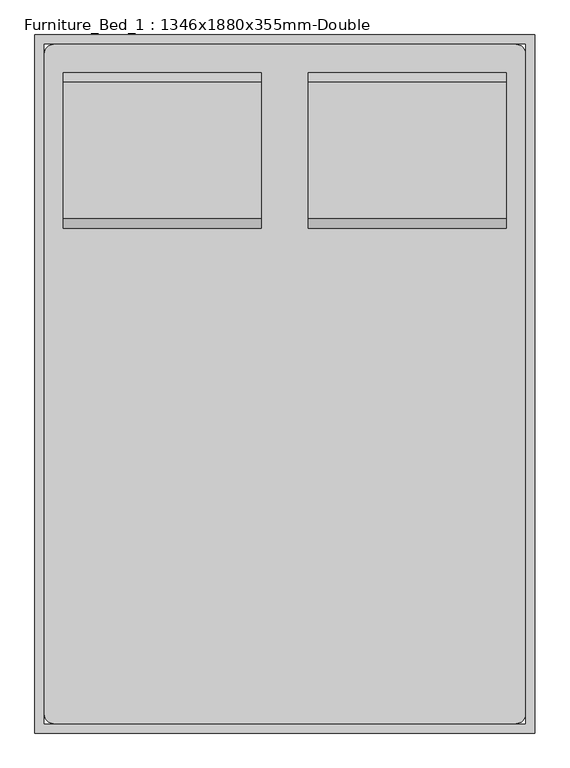
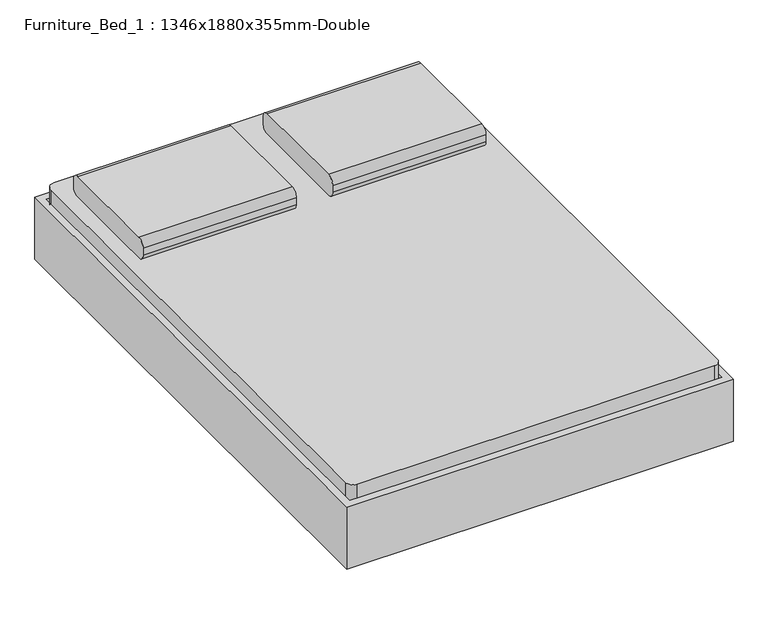
"""IFC4 building model written with IfcOpenShell, lengths in millimetres: furniture geometry, Furniture_Bed_1 : 1346x1880x355mm-Double."""

from ifc_helpers import new_model, si_unit, point, frame, frame_2d, origin, place, context, project, spatial, polyline, circle_curve, trimmed, segment, composite_curve, outline, extrude, source, transform, mapped, element, save
from ifc_brep_helpers import plane_surface, cylinder_surface, revolved_surface, advanced_brep


def furniture_bed_1_1346x1880x355mm_double_93dec6ea(model_context):
    return source(origin(), model_context, "Body", "SolidModel", [
        advanced_brep(
        [(-308.447541, -869.6295082, 196.85), (-308.447541, -869.6295082, 177.8), (-308.447541, -945.8295082, 177.8), (-308.447541, -945.8295082, 196.85), (-245.5113525, -869.6295082, 196.85), (-257.647541, -869.6295082, 177.8), (-257.647541, -945.8295082, 177.8), (-245.5113525, -945.8295082, 196.85), (-164.3115092, -869.6295082, 22.716374), (-181.5766725, -869.6295082, 14.6654962), (-181.5766725, -945.8295082, 14.6654962), (-164.3115092, -945.8295082, 22.716374), (-158.5564547, -869.6295082, 0.0), (-158.5564547, -869.6295082, 19.05), (-158.5564547, -945.8295082, 0.0), (-158.5564547, -945.8295082, 19.05), (-79.9439489, -869.6295082, 19.05), (-79.9439489, -869.6295082, 0.0), (-79.9439489, -945.8295082, 0.0), (-79.9439489, -945.8295082, 19.05), (-67.2439489, -869.6295082, 3.4029547), (-76.7689489, -869.6295082, 19.9007387), (-67.2439489, -945.8295082, 3.4029547), (-76.7689489, -945.8295082, 19.9007387), (-12.2513357, -869.6295082, 57.15), (-7.1469036, -869.6295082, 38.1), (-7.1469036, -945.8295082, 38.1), (-12.2513357, -945.8295082, 57.15), (690.5562537, -869.6295082, 57.15), (685.4518216, -869.6295082, 38.1), (685.4518216, -945.8295082, 38.1), (690.5562537, -945.8295082, 57.15), (755.0738669, -869.6295082, 19.9007387), (745.5488669, -869.6295082, 3.4029547), (745.5488669, -945.8295082, 3.4029547), (755.0738669, -945.8295082, 19.9007387), (758.2488669, -869.6295082, 0.0), (758.2488669, -869.6295082, 19.05), (758.2488669, -945.8295082, 0.0), (758.2488669, -945.8295082, 19.05), (836.8613728, -869.6295082, 19.05), (836.8613728, -869.6295082, 0.0), (836.8613728, -945.8295082, 0.0), (836.8613728, -945.8295082, 19.05), (859.8815906, -869.6295082, 14.6654962), (842.6164272, -869.6295082, 22.716374), (859.8815906, -945.8295082, 14.6654962), (842.6164272, -945.8295082, 22.716374), (923.8162705, -869.6295082, 196.85), (935.952459, -869.6295082, 177.8), (935.952459, -945.8295082, 177.8), (923.8162705, -945.8295082, 196.85), (986.752459, -869.6295082, 196.85), (986.752459, -945.8295082, 196.85), (986.752459, -945.8295082, 177.8), (986.752459, -869.6295082, 177.8)],
        [
            (0, 1),
            (1, 2),
            (2, 3),
            (3, 0),
            (0, 4),
            (4, 5),
            (5, 1),
            (5, 6),
            (6, 2),
            (6, 7),
            (7, 3),
            (7, 4),
            (4, 8),
            (8, 9),
            (9, 5),
            (9, 10),
            (10, 6),
            (10, 11),
            (11, 7),
            (11, 8),
            (12, 9, circle_curve(frame((-158.5564547, -869.6295082, 25.4), z_axis=(0.0, 1.0, 0.0), x_axis=(-0.9063077870366627, 0.0, -0.42261826174067213)), 25.4)),
            (8, 13, circle_curve(frame((-158.5564547, -869.6295082, 25.4), z_axis=(0.0, -1.0, 0.0), x_axis=(-0.9063077870366627, 0.0, -0.42261826174067213)), 6.35)),
            (13, 12),
            (14, 10, circle_curve(frame((-158.5564547, -945.8295082, 25.4), z_axis=(0.0, 1.0, 0.0), x_axis=(-0.9063077870366627, 0.0, -0.42261826174067213)), 25.4)),
            (12, 14),
            (15, 11, circle_curve(frame((-158.5564547, -945.8295082, 25.4), z_axis=(0.0, 1.0, 0.0), x_axis=(-0.9063077870366627, 0.0, -0.42261826174067213)), 6.35)),
            (14, 15),
            (15, 13),
            (13, 16),
            (16, 17),
            (17, 12),
            (17, 18),
            (18, 14),
            (18, 19),
            (19, 15),
            (19, 16),
            (20, 17, circle_curve(frame((-79.9439489, -869.6295082, 25.4), z_axis=(0.0, 1.0, 0.0), x_axis=(0.0, 0.0, -1.0)), 25.4)),
            (16, 21, circle_curve(frame((-79.9439489, -869.6295082, 25.4), z_axis=(0.0, -1.0, 0.0), x_axis=(0.0, 0.0, -1.0)), 6.35)),
            (21, 20),
            (22, 18, circle_curve(frame((-79.9439489, -945.8295082, 25.4), z_axis=(0.0, 1.0, 0.0), x_axis=(0.0, 0.0, -1.0)), 25.4)),
            (20, 22),
            (23, 19, circle_curve(frame((-79.9439489, -945.8295082, 25.4), z_axis=(0.0, 1.0, 0.0), x_axis=(0.0, 0.0, -1.0)), 6.35)),
            (22, 23),
            (23, 21),
            (21, 24),
            (24, 25),
            (25, 20),
            (25, 26),
            (26, 22),
            (26, 27),
            (27, 23),
            (27, 24),
            (24, 28),
            (28, 29),
            (29, 25),
            (29, 30),
            (30, 26),
            (30, 31),
            (31, 27),
            (31, 28),
            (28, 32),
            (32, 33),
            (33, 29),
            (33, 34),
            (34, 30),
            (34, 35),
            (35, 31),
            (35, 32),
            (36, 33, circle_curve(frame((758.2488669, -869.6295082, 25.4), z_axis=(0.0, 1.0, 0.0), x_axis=(-0.5000000000000486, 0.0, -0.8660254037844105)), 25.4)),
            (32, 37, circle_curve(frame((758.2488669, -869.6295082, 25.4), z_axis=(0.0, -1.0, 0.0), x_axis=(-0.5000000000000486, 0.0, -0.8660254037844105)), 6.35)),
            (37, 36),
            (38, 34, circle_curve(frame((758.2488669, -945.8295082, 25.4), z_axis=(0.0, 1.0, 0.0), x_axis=(-0.5000000000000486, 0.0, -0.8660254037844105)), 25.4)),
            (36, 38),
            (39, 35, circle_curve(frame((758.2488669, -945.8295082, 25.4), z_axis=(0.0, 1.0, 0.0), x_axis=(-0.5000000000000486, 0.0, -0.8660254037844105)), 6.35)),
            (38, 39),
            (39, 37),
            (37, 40),
            (40, 41),
            (41, 36),
            (41, 42),
            (42, 38),
            (42, 43),
            (43, 39),
            (43, 40),
            (44, 41, circle_curve(frame((836.8613728, -869.6295082, 25.4), z_axis=(0.0, 1.0, 0.0), x_axis=(0.0, 0.0, -1.0)), 25.4)),
            (40, 45, circle_curve(frame((836.8613728, -869.6295082, 25.4), z_axis=(0.0, -1.0, 0.0), x_axis=(0.0, 0.0, -1.0)), 6.35)),
            (45, 44),
            (46, 42, circle_curve(frame((836.8613728, -945.8295082, 25.4), z_axis=(0.0, 1.0, 0.0), x_axis=(0.0, 0.0, -1.0)), 25.4)),
            (44, 46),
            (47, 43, circle_curve(frame((836.8613728, -945.8295082, 25.4), z_axis=(0.0, 1.0, 0.0), x_axis=(0.0, 0.0, -1.0)), 6.35)),
            (46, 47),
            (47, 45),
            (45, 48),
            (48, 49),
            (49, 44),
            (49, 50),
            (50, 46),
            (50, 51),
            (51, 47),
            (51, 48),
            (52, 53),
            (53, 54),
            (54, 55),
            (55, 52),
            (48, 52),
            (55, 49),
            (54, 50),
            (53, 51),
        ],
        [
            plane_surface(frame((-308.447541, -1174.4295082, -127.5947323), z_axis=(-1.0, 0.0, 0.0), x_axis=(0.0, 1.0, 0.0))),
            plane_surface(frame((-308.447541, -869.6295082, 196.85), z_axis=(0.0, 1.0, 0.0), x_axis=(1.0, 0.0, 0.0))),
            plane_surface(frame((-308.447541, -869.6295082, 177.8), z_axis=(0.0, 0.0, -1.0), x_axis=(1.0, 0.0, 0.0))),
            plane_surface(frame((-308.447541, -945.8295082, 177.8), z_axis=(0.0, -1.0, 0.0), x_axis=(1.0, 0.0, 0.0))),
            plane_surface(frame((-308.447541, -945.8295082, 196.85), z_axis=(0.0, 0.0, 1.0), x_axis=(1.0, 0.0, 0.0))),
            plane_surface(frame((-245.5113525, -869.6295082, 196.85), z_axis=(0.0, 1.0, 0.0), x_axis=(0.42261826174067146, 0.0, -0.906307787036663))),
            plane_surface(frame((-257.647541, -869.6295082, 177.8), z_axis=(-0.9063077870366631, 0.0, -0.4226182617406713), x_axis=(0.4226182617406713, 0.0, -0.9063077870366631))),
            plane_surface(frame((-257.647541, -945.8295082, 177.8), z_axis=(0.0, -1.0, 0.0), x_axis=(0.4226182617406716, 0.0, -0.9063077870366629))),
            plane_surface(frame((-245.5113525, -945.8295082, 196.85), z_axis=(0.906307787036663, 0.0, 0.4226182617406716), x_axis=(0.4226182617406716, 0.0, -0.906307787036663))),
            plane_surface(frame((-158.5564547, -869.6295082, 25.4), z_axis=(0.0, 1.0, 0.0), x_axis=(-0.9063077870366627, 0.0, -0.42261826174067213))),
            cylinder_surface(frame((-158.5564547, -1174.4295082, 25.4), z_axis=(0.0, -1.0, 0.0), x_axis=(-0.9063077870366627, 0.0, -0.42261826174067213)), 25.4),
            plane_surface(frame((-158.5564547, -945.8295082, 25.4), z_axis=(0.0, -1.0, 0.0), x_axis=(-0.9063077870366627, 0.0, -0.42261826174067213))),
            revolved_surface(polyline([(-164.31150914768278, -945.8295082, 22.716374037946732), (-164.31150914768278, -869.6295082, 22.716374037946732)]), (-158.5564547, -1174.4295082, 25.4), (0.0, -1.0, 0.0)),
            plane_surface(frame((-158.5564547, -869.6295082, 19.05), z_axis=(0.0, 1.0, 0.0), x_axis=(1.0, 0.0, 0.0))),
            plane_surface(frame((-158.5564547, -869.6295082, 0.0), z_axis=(0.0, 0.0, -1.0), x_axis=(1.0, 0.0, 0.0))),
            plane_surface(frame((-158.5564547, -945.8295082, 0.0), z_axis=(0.0, -1.0, 0.0), x_axis=(1.0, 0.0, 0.0))),
            plane_surface(frame((-158.5564547, -945.8295082, 19.05), z_axis=(0.0, 0.0, 1.0), x_axis=(1.0, 0.0, 0.0))),
            plane_surface(frame((-79.9439489, -869.6295082, 25.4), z_axis=(0.0, 1.0, 0.0), x_axis=(0.0, 0.0, -1.0))),
            cylinder_surface(frame((-79.9439489, -1174.4295082, 25.4), z_axis=(0.0, -1.0, 0.0), x_axis=(0.0, 0.0, -1.0)), 25.4),
            plane_surface(frame((-79.9439489, -945.8295082, 25.4), z_axis=(0.0, -1.0, 0.0), x_axis=(0.0, 0.0, -1.0))),
            revolved_surface(polyline([(-79.9439489, -945.8295082, 19.049999999999997), (-79.9439489, -869.6295082, 19.049999999999997)]), (-79.9439489, -1174.4295082, 25.4), (0.0, -1.0, 0.0)),
            plane_surface(frame((-76.7689489, -869.6295082, 19.9007387), z_axis=(0.0, 1.0, 0.0), x_axis=(0.8660254037844782, 0.0, 0.4999999999999314))),
            plane_surface(frame((-67.2439489, -869.6295082, 3.4029547), z_axis=(0.49999999999993133, 0.0, -0.8660254037844783), x_axis=(0.8660254037844783, 0.0, 0.49999999999993133))),
            plane_surface(frame((-67.2439489, -945.8295082, 3.4029547), z_axis=(0.0, -1.0, 0.0), x_axis=(0.8660254037844785, 0.0, 0.499999999999931))),
            plane_surface(frame((-76.7689489, -945.8295082, 19.9007387), z_axis=(-0.49999999999993144, 0.0, 0.8660254037844782), x_axis=(0.8660254037844782, 0.0, 0.49999999999993144))),
            plane_surface(frame((-12.2513357, -869.6295082, 57.15), z_axis=(0.0, 1.0, 0.0), x_axis=(1.0, 0.0, 0.0))),
            plane_surface(frame((-7.1469036, -869.6295082, 38.1), z_axis=(0.0, 0.0, -1.0), x_axis=(1.0, 0.0, 0.0))),
            plane_surface(frame((-7.1469036, -945.8295082, 38.1), z_axis=(0.0, -1.0, 0.0), x_axis=(1.0, 0.0, 0.0))),
            plane_surface(frame((-12.2513357, -945.8295082, 57.15), z_axis=(0.0, 0.0, 1.0), x_axis=(1.0, 0.0, 0.0))),
            plane_surface(frame((690.5562537, -869.6295082, 57.15), z_axis=(0.0, 1.0, 0.0), x_axis=(0.8660254037844104, 0.0, -0.5000000000000491))),
            plane_surface(frame((685.4518216, -869.6295082, 38.1), z_axis=(-0.5000000000000484, 0.0, -0.8660254037844108), x_axis=(0.8660254037844108, 0.0, -0.5000000000000484))),
            plane_surface(frame((685.4518216, -945.8295082, 38.1), z_axis=(0.0, -1.0000000000000002, 0.0), x_axis=(0.8660254037844103, 0.0, -0.5000000000000493))),
            plane_surface(frame((690.5562537, -945.8295082, 57.15), z_axis=(0.5000000000000485, 0.0, 0.8660254037844106), x_axis=(0.8660254037844106, 0.0, -0.5000000000000485))),
            plane_surface(frame((758.2488669, -869.6295082, 25.4), z_axis=(0.0, 1.0000000000000002, 0.0), x_axis=(-0.5000000000000487, 0.0, -0.8660254037844106))),
            cylinder_surface(frame((758.2488669, -1174.4295082, 25.4), z_axis=(0.0, -1.0, 0.0), x_axis=(-0.5000000000000486, 0.0, -0.8660254037844105)), 25.4),
            plane_surface(frame((758.2488669, -945.8295082, 25.4), z_axis=(0.0, -1.0000000000000002, 0.0), x_axis=(-0.5000000000000487, 0.0, -0.8660254037844106))),
            revolved_surface(polyline([(755.0738668999998, -945.8295082, 19.900738685968992), (755.0738668999998, -869.6295082, 19.900738685968992)]), (758.2488669, -1174.4295082, 25.4), (0.0, -1.0, 0.0)),
            plane_surface(frame((758.2488669, -869.6295082, 19.05), z_axis=(0.0, 1.0, 0.0), x_axis=(1.0, 0.0, 0.0))),
            plane_surface(frame((758.2488669, -869.6295082, 0.0), z_axis=(0.0, 0.0, -1.0), x_axis=(1.0, 0.0, 0.0))),
            plane_surface(frame((758.2488669, -945.8295082, 0.0), z_axis=(0.0, -1.0, 0.0), x_axis=(1.0, 0.0, 0.0))),
            plane_surface(frame((758.2488669, -945.8295082, 19.05), z_axis=(0.0, 0.0, 1.0), x_axis=(1.0, 0.0, 0.0))),
            plane_surface(frame((836.8613728, -869.6295082, 25.4), z_axis=(0.0, 1.0, 0.0), x_axis=(0.0, 0.0, -1.0))),
            cylinder_surface(frame((836.8613728, -1174.4295082, 25.4), z_axis=(0.0, -1.0, 0.0), x_axis=(0.0, 0.0, -1.0)), 25.4),
            plane_surface(frame((836.8613728, -945.8295082, 25.4), z_axis=(0.0, -1.0, 0.0), x_axis=(0.0, 0.0, -1.0))),
            revolved_surface(polyline([(836.8613728, -945.8295082, 19.049999999999997), (836.8613728, -869.6295082, 19.049999999999997)]), (836.8613728, -1174.4295082, 25.4), (0.0, -1.0, 0.0)),
            plane_surface(frame((842.6164272, -869.6295082, 22.716374), z_axis=(0.0, 1.0, 0.0), x_axis=(0.4226182617405402, 0.0, 0.9063077870367242))),
            plane_surface(frame((859.8815906, -869.6295082, 14.6654962), z_axis=(0.9063077870367245, 0.0, -0.42261826174053974), x_axis=(0.42261826174053974, 0.0, 0.9063077870367245))),
            plane_surface(frame((859.8815906, -945.8295082, 14.6654962), z_axis=(0.0, -1.0000000000000002, 0.0), x_axis=(0.42261826174053974, 0.0, 0.9063077870367245))),
            plane_surface(frame((842.6164272, -945.8295082, 22.716374), z_axis=(-0.9063077870367247, 0.0, 0.4226182617405394), x_axis=(0.4226182617405394, 0.0, 0.9063077870367247))),
            plane_surface(frame((986.752459, -1174.4295082, -127.5947323), z_axis=(1.0, 0.0, 0.0), x_axis=(0.0, 1.0, 0.0))),
            plane_surface(frame((923.8162705, -869.6295082, 196.85), z_axis=(0.0, 1.0, 0.0), x_axis=(1.0, 0.0, 0.0))),
            plane_surface(frame((935.952459, -869.6295082, 177.8), z_axis=(0.0, 0.0, -1.0), x_axis=(1.0, 0.0, 0.0))),
            plane_surface(frame((935.952459, -945.8295082, 177.8), z_axis=(0.0, -1.0, 0.0), x_axis=(1.0, 0.0, 0.0))),
            plane_surface(frame((923.8162705, -945.8295082, 196.85), z_axis=(0.0, 0.0, 1.0), x_axis=(1.0, 0.0, 0.0))),
        ],
        [
            (0, [[1, 2, 3, 4]]),
            (1, [[-1, 5, 6, 7]]),
            (2, [[-2, -7, 8, 9]]),
            (3, [[-3, -9, 10, 11]]),
            (4, [[-4, -11, 12, -5]]),
            (5, [[-6, 13, 14, 15]]),
            (6, [[-8, -15, 16, 17]]),
            (7, [[-10, -17, 18, 19]]),
            (8, [[-12, -19, 20, -13]]),
            (9, [[21, -14, 22, 23]]),
            (10, [[24, -16, -21, 25]]),
            (11, [[26, -18, -24, 27]]),
            (12, [[-22, -20, -26, 28]]),
            (13, [[-23, 29, 30, 31]]),
            (14, [[-25, -31, 32, 33]]),
            (15, [[-27, -33, 34, 35]]),
            (16, [[-28, -35, 36, -29]]),
            (17, [[37, -30, 38, 39]]),
            (18, [[40, -32, -37, 41]]),
            (19, [[42, -34, -40, 43]]),
            (20, [[-38, -36, -42, 44]]),
            (21, [[-39, 45, 46, 47]]),
            (22, [[-41, -47, 48, 49]]),
            (23, [[-43, -49, 50, 51]]),
            (24, [[-44, -51, 52, -45]]),
            (25, [[-46, 53, 54, 55]]),
            (26, [[-48, -55, 56, 57]]),
            (27, [[-50, -57, 58, 59]]),
            (28, [[-52, -59, 60, -53]]),
            (29, [[-54, 61, 62, 63]]),
            (30, [[-56, -63, 64, 65]]),
            (31, [[-58, -65, 66, 67]]),
            (32, [[-60, -67, 68, -61]]),
            (33, [[69, -62, 70, 71]]),
            (34, [[72, -64, -69, 73]]),
            (35, [[74, -66, -72, 75]]),
            (36, [[-70, -68, -74, 76]]),
            (37, [[-71, 77, 78, 79]]),
            (38, [[-73, -79, 80, 81]]),
            (39, [[-75, -81, 82, 83]]),
            (40, [[-76, -83, 84, -77]]),
            (41, [[85, -78, 86, 87]]),
            (42, [[88, -80, -85, 89]]),
            (43, [[90, -82, -88, 91]]),
            (44, [[-86, -84, -90, 92]]),
            (45, [[-87, 93, 94, 95]]),
            (46, [[-89, -95, 96, 97]]),
            (47, [[-91, -97, 98, 99]]),
            (48, [[-92, -99, 100, -93]]),
            (49, [[101, 102, 103, 104]]),
            (50, [[-94, 105, -104, 106]]),
            (51, [[-96, -106, -103, 107]]),
            (52, [[-98, -107, -102, 108]]),
            (53, [[-100, -108, -101, -105]]),
        ],
    ),
        extrude(outline(composite_curve([segment(polyline([(-283.047541, 680.1704918), (961.352459, 680.1704918)]), True, "CONTINUOUS"), segment(trimmed(circle_curve(frame_2d((961.352459, 654.7704918)), 25.4), [point((961.352459, 680.1704918))], [point((986.752459, 654.7704918))], False, "CARTESIAN"), True, "CONTINUOUS"), segment(polyline([(986.752459, 654.7704918), (986.752459, -1123.6295082)]), True, "CONTINUOUS"), segment(trimmed(circle_curve(frame_2d((961.352459, -1123.6295082)), 25.4), [point((986.752459, -1123.6295082))], [point((961.352459, -1149.0295082))], False, "CARTESIAN"), True, "CONTINUOUS"), segment(polyline([(961.352459, -1149.0295082), (-283.047541, -1149.0295082)]), True, "CONTINUOUS"), segment(trimmed(circle_curve(frame_2d((-283.047541, -1123.6295082)), 25.4), [point((-283.047541, -1149.0295082))], [point((-308.447541, -1123.6295082))], False, "CARTESIAN"), True, "CONTINUOUS"), segment(polyline([(-308.447541, -1123.6295082), (-308.447541, 654.7704918)]), True, "CONTINUOUS"), segment(trimmed(circle_curve(frame_2d((-283.047541, 654.7704918)), 25.4), [point((-308.447541, 654.7704918))], [point((-283.047541, 680.1704918))], False, "CARTESIAN"), True, "CONTINUOUS")], self_intersect=False)), frame((0.0, 0.0, 203.2), z_axis=(0.0, 0.0, 1.0), x_axis=(1.0, 0.0, 0.0)), (0.0, 0.0, 1.0), 203.2),
        advanced_brep(
        [(-308.1231784, 451.5704918, 177.8), (-308.1231784, 375.3704918, 177.8), (-308.1231784, 375.3704918, 196.85), (-308.1231784, 451.5704918, 196.85), (-257.3231784, 451.5704918, 177.8), (-257.3231784, 375.3704918, 177.8), (-245.1869899, 375.3704918, 196.85), (-245.1869899, 451.5704918, 196.85), (-181.2523099, 451.5704918, 14.6654962), (-181.2523099, 375.3704918, 14.6654962), (-163.9871466, 375.3704918, 22.716374), (-163.9871466, 451.5704918, 22.716374), (-158.2320921, 375.3704918, 0.0), (-158.2320921, 451.5704918, 0.0), (-158.2320921, 375.3704918, 19.05), (-158.2320921, 451.5704918, 19.05), (-79.6195862, 451.5704918, 0.0), (-79.6195862, 375.3704918, 0.0), (-79.6195862, 375.3704918, 19.05), (-79.6195862, 451.5704918, 19.05), (-66.9195862, 375.3704918, 3.4029547), (-66.9195862, 451.5704918, 3.4029547), (-76.4445862, 375.3704918, 19.9007387), (-76.4445862, 451.5704918, 19.9007387), (-6.822541, 451.5704918, 38.1), (-6.822541, 375.3704918, 38.1), (-11.9269731, 375.3704918, 57.15), (-11.9269731, 451.5704918, 57.15), (685.4518216, 451.5704918, 38.1), (685.4518216, 375.3704918, 38.1), (690.5562537, 375.3704918, 57.15), (690.5562537, 451.5704918, 57.15), (745.5488669, 451.5704918, 3.4029547), (745.5488669, 375.3704918, 3.4029547), (755.0738669, 375.3704918, 19.9007387), (755.0738669, 451.5704918, 19.9007387), (758.2488669, 375.3704918, 0.0), (758.2488669, 451.5704918, 0.0), (758.2488669, 375.3704918, 19.05), (758.2488669, 451.5704918, 19.05), (836.8613728, 451.5704918, 0.0), (836.8613728, 375.3704918, 0.0), (836.8613728, 375.3704918, 19.05), (836.8613728, 451.5704918, 19.05), (859.8815906, 375.3704918, 14.6654962), (859.8815906, 451.5704918, 14.6654962), (842.6164272, 375.3704918, 22.716374), (842.6164272, 451.5704918, 22.716374), (935.952459, 451.5704918, 177.8), (935.952459, 375.3704918, 177.8), (923.8162705, 375.3704918, 196.85), (923.8162705, 451.5704918, 196.85), (986.752459, 451.5704918, 177.8), (986.752459, 451.5704918, 196.85), (986.752459, 375.3704918, 196.85), (986.752459, 375.3704918, 177.8)],
        [
            (0, 1),
            (1, 2),
            (2, 3),
            (3, 0),
            (0, 4),
            (4, 5),
            (5, 1),
            (5, 6),
            (6, 2),
            (6, 7),
            (7, 3),
            (7, 4),
            (4, 8),
            (8, 9),
            (9, 5),
            (9, 10),
            (10, 6),
            (10, 11),
            (11, 7),
            (11, 8),
            (12, 9, circle_curve(frame((-158.2320921, 375.3704918, 25.4), z_axis=(0.0, 1.0, 0.0), x_axis=(-0.906307787036649, 0.0, -0.4226182617407015)), 25.4)),
            (8, 13, circle_curve(frame((-158.2320921, 451.5704918, 25.4), z_axis=(0.0, -1.0, 0.0), x_axis=(-0.906307787036649, 0.0, -0.4226182617407015)), 25.4)),
            (13, 12),
            (14, 10, circle_curve(frame((-158.2320921, 375.3704918, 25.4), z_axis=(0.0, 1.0, 0.0), x_axis=(-0.906307787036649, 0.0, -0.4226182617407015)), 6.35)),
            (12, 14),
            (15, 11, circle_curve(frame((-158.2320921, 451.5704918, 25.4), z_axis=(0.0, 1.0, 0.0), x_axis=(-0.906307787036649, 0.0, -0.4226182617407015)), 6.35)),
            (14, 15),
            (15, 13),
            (13, 16),
            (16, 17),
            (17, 12),
            (17, 18),
            (18, 14),
            (18, 19),
            (19, 15),
            (19, 16),
            (20, 17, circle_curve(frame((-79.6195862, 375.3704918, 25.4), z_axis=(0.0, 1.0, 0.0), x_axis=(0.0, 0.0, -1.0)), 25.4)),
            (16, 21, circle_curve(frame((-79.6195862, 451.5704918, 25.4), z_axis=(0.0, -1.0, 0.0), x_axis=(0.0, 0.0, -1.0)), 25.4)),
            (21, 20),
            (22, 18, circle_curve(frame((-79.6195862, 375.3704918, 25.4), z_axis=(0.0, 1.0, 0.0), x_axis=(0.0, 0.0, -1.0)), 6.35)),
            (20, 22),
            (23, 19, circle_curve(frame((-79.6195862, 451.5704918, 25.4), z_axis=(0.0, 1.0, 0.0), x_axis=(0.0, 0.0, -1.0)), 6.35)),
            (22, 23),
            (23, 21),
            (21, 24),
            (24, 25),
            (25, 20),
            (25, 26),
            (26, 22),
            (26, 27),
            (27, 23),
            (27, 24),
            (24, 28),
            (28, 29),
            (29, 25),
            (29, 30),
            (30, 26),
            (30, 31),
            (31, 27),
            (31, 28),
            (28, 32),
            (32, 33),
            (33, 29),
            (33, 34),
            (34, 30),
            (34, 35),
            (35, 31),
            (35, 32),
            (36, 33, circle_curve(frame((758.2488669, 375.3704918, 25.4), z_axis=(0.0, 1.0, 0.0), x_axis=(-0.5000000000000444, 0.0, -0.866025403784413)), 25.4)),
            (32, 37, circle_curve(frame((758.2488669, 451.5704918, 25.4), z_axis=(0.0, -1.0, 0.0), x_axis=(-0.5000000000000444, 0.0, -0.866025403784413)), 25.4)),
            (37, 36),
            (38, 34, circle_curve(frame((758.2488669, 375.3704918, 25.4), z_axis=(0.0, 1.0, 0.0), x_axis=(-0.5000000000000444, 0.0, -0.866025403784413)), 6.35)),
            (36, 38),
            (39, 35, circle_curve(frame((758.2488669, 451.5704918, 25.4), z_axis=(0.0, 1.0, 0.0), x_axis=(-0.5000000000000444, 0.0, -0.866025403784413)), 6.35)),
            (38, 39),
            (39, 37),
            (37, 40),
            (40, 41),
            (41, 36),
            (41, 42),
            (42, 38),
            (42, 43),
            (43, 39),
            (43, 40),
            (44, 41, circle_curve(frame((836.8613728, 375.3704918, 25.4), z_axis=(0.0, 1.0, 0.0), x_axis=(0.0, 0.0, -1.0)), 25.4)),
            (40, 45, circle_curve(frame((836.8613728, 451.5704918, 25.4), z_axis=(0.0, -1.0, 0.0), x_axis=(0.0, 0.0, -1.0)), 25.4)),
            (45, 44),
            (46, 42, circle_curve(frame((836.8613728, 375.3704918, 25.4), z_axis=(0.0, 1.0, 0.0), x_axis=(0.0, 0.0, -1.0)), 6.35)),
            (44, 46),
            (47, 43, circle_curve(frame((836.8613728, 451.5704918, 25.4), z_axis=(0.0, 1.0, 0.0), x_axis=(0.0, 0.0, -1.0)), 6.35)),
            (46, 47),
            (47, 45),
            (45, 48),
            (48, 49),
            (49, 44),
            (49, 50),
            (50, 46),
            (50, 51),
            (51, 47),
            (51, 48),
            (52, 53),
            (53, 54),
            (54, 55),
            (55, 52),
            (48, 52),
            (55, 49),
            (54, 50),
            (53, 51),
        ],
        [
            plane_surface(frame((-308.1231784, 705.5704918, -152.9490627), z_axis=(-1.0, 0.0, 0.0), x_axis=(0.0, 1.0, 0.0))),
            plane_surface(frame((-308.1231784, 451.5704918, 177.8), z_axis=(0.0, 0.0, -1.0), x_axis=(1.0, 0.0, 0.0))),
            plane_surface(frame((-308.1231784, 375.3704918, 177.8), z_axis=(0.0, -1.0, 0.0), x_axis=(1.0, 0.0, 0.0))),
            plane_surface(frame((-308.1231784, 375.3704918, 196.85), z_axis=(0.0, 0.0, 1.0), x_axis=(1.0, 0.0, 0.0))),
            plane_surface(frame((-308.1231784, 451.5704918, 196.85), z_axis=(0.0, 1.0, 0.0), x_axis=(1.0, 0.0, 0.0))),
            plane_surface(frame((-257.3231784, 451.5704918, 177.8), z_axis=(-0.9063077870366483, 0.0, -0.4226182617407031), x_axis=(0.4226182617407031, 0.0, -0.9063077870366483))),
            plane_surface(frame((-257.3231784, 375.3704918, 177.8), z_axis=(0.0, -1.0, 0.0), x_axis=(0.4226182617407027, 0.0, -0.9063077870366485))),
            plane_surface(frame((-245.1869899, 375.3704918, 196.85), z_axis=(0.9063077870366484, 0.0, 0.4226182617407029), x_axis=(0.4226182617407029, 0.0, -0.9063077870366484))),
            plane_surface(frame((-245.1869899, 451.5704918, 196.85), z_axis=(0.0, 1.0, 0.0), x_axis=(0.4226182617407027, 0.0, -0.9063077870366485))),
            cylinder_surface(frame((-158.2320921, 705.5704918, 25.4), z_axis=(0.0, -1.0, 0.0), x_axis=(-0.906307787036649, 0.0, -0.4226182617407015)), 25.4),
            plane_surface(frame((-158.2320921, 375.3704918, 25.4), z_axis=(0.0, -1.0, 0.0), x_axis=(-0.906307787036649, 0.0, -0.4226182617407015))),
            revolved_surface(polyline([(-163.9871465476827, 375.3704918, 22.716374037946544), (-163.9871465476827, 451.5704918, 22.716374037946544)]), (-158.2320921, 705.5704918, 25.4), (0.0, -1.0, 0.0)),
            plane_surface(frame((-158.2320921, 451.5704918, 25.4), z_axis=(0.0, 1.0, 0.0), x_axis=(-0.906307787036649, 0.0, -0.4226182617407015))),
            plane_surface(frame((-158.2320921, 451.5704918, 0.0), z_axis=(0.0, 0.0, -1.0), x_axis=(1.0, 0.0, 0.0))),
            plane_surface(frame((-158.2320921, 375.3704918, 0.0), z_axis=(0.0, -1.0, 0.0), x_axis=(1.0, 0.0, 0.0))),
            plane_surface(frame((-158.2320921, 375.3704918, 19.05), z_axis=(0.0, 0.0, 1.0), x_axis=(1.0, 0.0, 0.0))),
            plane_surface(frame((-158.2320921, 451.5704918, 19.05), z_axis=(0.0, 1.0, 0.0), x_axis=(1.0, 0.0, 0.0))),
            cylinder_surface(frame((-79.6195862, 705.5704918, 25.4), z_axis=(0.0, -1.0, 0.0), x_axis=(0.0, 0.0, -1.0)), 25.4),
            plane_surface(frame((-79.6195862, 375.3704918, 25.4), z_axis=(0.0, -1.0, 0.0), x_axis=(0.0, 0.0, -1.0))),
            revolved_surface(polyline([(-79.6195862, 375.3704918, 19.049999999999997), (-79.6195862, 451.5704918, 19.049999999999997)]), (-79.6195862, 705.5704918, 25.4), (0.0, -1.0, 0.0)),
            plane_surface(frame((-79.6195862, 451.5704918, 25.4), z_axis=(0.0, 1.0, 0.0), x_axis=(0.0, 0.0, -1.0))),
            plane_surface(frame((-66.9195862, 451.5704918, 3.4029547), z_axis=(0.4999999999998771, 0.0, -0.8660254037845097), x_axis=(0.8660254037845097, 0.0, 0.4999999999998771))),
            plane_surface(frame((-66.9195862, 375.3704918, 3.4029547), z_axis=(0.0, -1.0000000000000002, 0.0), x_axis=(0.8660254037845102, 0.0, 0.49999999999987627))),
            plane_surface(frame((-76.4445862, 375.3704918, 19.9007387), z_axis=(-0.49999999999987643, 0.0, 0.86602540378451), x_axis=(0.86602540378451, 0.0, 0.49999999999987643))),
            plane_surface(frame((-76.4445862, 451.5704918, 19.9007387), z_axis=(0.0, 1.0, 0.0), x_axis=(0.8660254037845102, 0.0, 0.4999999999998761))),
            plane_surface(frame((-6.822541, 451.5704918, 38.1), z_axis=(0.0, 0.0, -1.0), x_axis=(1.0, 0.0, 0.0))),
            plane_surface(frame((-6.822541, 375.3704918, 38.1), z_axis=(0.0, -1.0, 0.0), x_axis=(1.0, 0.0, 0.0))),
            plane_surface(frame((-11.9269731, 375.3704918, 57.15), z_axis=(0.0, 0.0, 1.0), x_axis=(1.0, 0.0, 0.0))),
            plane_surface(frame((-11.9269731, 451.5704918, 57.15), z_axis=(0.0, 1.0, 0.0), x_axis=(1.0, 0.0, 0.0))),
            plane_surface(frame((685.4518216, 451.5704918, 38.1), z_axis=(-0.5000000000000445, 0.0, -0.866025403784413), x_axis=(0.866025403784413, 0.0, -0.5000000000000445))),
            plane_surface(frame((685.4518216, 375.3704918, 38.1), z_axis=(0.0, -1.0, 0.0), x_axis=(0.8660254037844118, 0.0, -0.5000000000000464))),
            plane_surface(frame((690.5562537, 375.3704918, 57.15), z_axis=(0.5000000000000461, 0.0, 0.8660254037844121), x_axis=(0.8660254037844121, 0.0, -0.5000000000000461))),
            plane_surface(frame((690.5562537, 451.5704918, 57.15), z_axis=(0.0, 1.0, 0.0), x_axis=(0.8660254037844126, 0.0, -0.5000000000000452))),
            cylinder_surface(frame((758.2488669, 705.5704918, 25.4), z_axis=(0.0, -1.0, 0.0), x_axis=(-0.5000000000000444, 0.0, -0.866025403784413)), 25.4),
            plane_surface(frame((758.2488669, 375.3704918, 25.4), z_axis=(0.0, -1.0000000000000002, 0.0), x_axis=(-0.5000000000000445, 0.0, -0.8660254037844131))),
            revolved_surface(polyline([(755.0738668999998, 375.3704918, 19.900738685968975), (755.0738668999998, 451.5704918, 19.900738685968975)]), (758.2488669, 705.5704918, 25.4), (0.0, -1.0, 0.0)),
            plane_surface(frame((758.2488669, 451.5704918, 25.4), z_axis=(0.0, 1.0000000000000002, 0.0), x_axis=(-0.5000000000000445, 0.0, -0.8660254037844131))),
            plane_surface(frame((758.2488669, 451.5704918, 0.0), z_axis=(0.0, 0.0, -1.0), x_axis=(1.0, 0.0, 0.0))),
            plane_surface(frame((758.2488669, 375.3704918, 0.0), z_axis=(0.0, -1.0, 0.0), x_axis=(1.0, 0.0, 0.0))),
            plane_surface(frame((758.2488669, 375.3704918, 19.05), z_axis=(0.0, 0.0, 1.0), x_axis=(1.0, 0.0, 0.0))),
            plane_surface(frame((758.2488669, 451.5704918, 19.05), z_axis=(0.0, 1.0, 0.0), x_axis=(1.0, 0.0, 0.0))),
            cylinder_surface(frame((836.8613728, 705.5704918, 25.4), z_axis=(0.0, -1.0, 0.0), x_axis=(0.0, 0.0, -1.0)), 25.4),
            plane_surface(frame((836.8613728, 375.3704918, 25.4), z_axis=(0.0, -1.0, 0.0), x_axis=(0.0, 0.0, -1.0))),
            revolved_surface(polyline([(836.8613728, 375.3704918, 19.049999999999997), (836.8613728, 451.5704918, 19.049999999999997)]), (836.8613728, 705.5704918, 25.4), (0.0, -1.0, 0.0)),
            plane_surface(frame((836.8613728, 451.5704918, 25.4), z_axis=(0.0, 1.0, 0.0), x_axis=(0.0, 0.0, -1.0))),
            plane_surface(frame((859.8815906, 451.5704918, 14.6654962), z_axis=(0.9063077870366807, 0.0, -0.42261826174063377), x_axis=(0.42261826174063377, 0.0, 0.9063077870366807))),
            plane_surface(frame((859.8815906, 375.3704918, 14.6654962), z_axis=(0.0, -1.0, 0.0), x_axis=(0.422618261740633, 0.0, 0.9063077870366809))),
            plane_surface(frame((842.6164272, 375.3704918, 22.716374), z_axis=(-0.9063077870366809, 0.0, 0.4226182617406331), x_axis=(0.4226182617406331, 0.0, 0.9063077870366809))),
            plane_surface(frame((842.6164272, 451.5704918, 22.716374), z_axis=(0.0, 1.0, 0.0), x_axis=(0.42261826174063294, 0.0, 0.906307787036681))),
            plane_surface(frame((986.752459, 705.5704918, -152.9490627), z_axis=(1.0, 0.0, 0.0), x_axis=(0.0, 1.0, 0.0))),
            plane_surface(frame((935.952459, 451.5704918, 177.8), z_axis=(0.0, 0.0, -1.0), x_axis=(1.0, 0.0, 0.0))),
            plane_surface(frame((935.952459, 375.3704918, 177.8), z_axis=(0.0, -1.0, 0.0), x_axis=(1.0, 0.0, 0.0))),
            plane_surface(frame((923.8162705, 375.3704918, 196.85), z_axis=(0.0, 0.0, 1.0), x_axis=(1.0, 0.0, 0.0))),
            plane_surface(frame((923.8162705, 451.5704918, 196.85), z_axis=(0.0, 1.0, 0.0), x_axis=(1.0, 0.0, 0.0))),
        ],
        [
            (0, [[1, 2, 3, 4]]),
            (1, [[-1, 5, 6, 7]]),
            (2, [[-2, -7, 8, 9]]),
            (3, [[-3, -9, 10, 11]]),
            (4, [[-4, -11, 12, -5]]),
            (5, [[-6, 13, 14, 15]]),
            (6, [[-8, -15, 16, 17]]),
            (7, [[-10, -17, 18, 19]]),
            (8, [[-12, -19, 20, -13]]),
            (9, [[21, -14, 22, 23]]),
            (10, [[24, -16, -21, 25]]),
            (11, [[26, -18, -24, 27]]),
            (12, [[-22, -20, -26, 28]]),
            (13, [[-23, 29, 30, 31]]),
            (14, [[-25, -31, 32, 33]]),
            (15, [[-27, -33, 34, 35]]),
            (16, [[-28, -35, 36, -29]]),
            (17, [[37, -30, 38, 39]]),
            (18, [[40, -32, -37, 41]]),
            (19, [[42, -34, -40, 43]]),
            (20, [[-38, -36, -42, 44]]),
            (21, [[-39, 45, 46, 47]]),
            (22, [[-41, -47, 48, 49]]),
            (23, [[-43, -49, 50, 51]]),
            (24, [[-44, -51, 52, -45]]),
            (25, [[-46, 53, 54, 55]]),
            (26, [[-48, -55, 56, 57]]),
            (27, [[-50, -57, 58, 59]]),
            (28, [[-52, -59, 60, -53]]),
            (29, [[-54, 61, 62, 63]]),
            (30, [[-56, -63, 64, 65]]),
            (31, [[-58, -65, 66, 67]]),
            (32, [[-60, -67, 68, -61]]),
            (33, [[69, -62, 70, 71]]),
            (34, [[72, -64, -69, 73]]),
            (35, [[74, -66, -72, 75]]),
            (36, [[-70, -68, -74, 76]]),
            (37, [[-71, 77, 78, 79]]),
            (38, [[-73, -79, 80, 81]]),
            (39, [[-75, -81, 82, 83]]),
            (40, [[-76, -83, 84, -77]]),
            (41, [[85, -78, 86, 87]]),
            (42, [[88, -80, -85, 89]]),
            (43, [[90, -82, -88, 91]]),
            (44, [[-86, -84, -90, 92]]),
            (45, [[-87, 93, 94, 95]]),
            (46, [[-89, -95, 96, 97]]),
            (47, [[-91, -97, 98, 99]]),
            (48, [[-92, -99, 100, -93]]),
            (49, [[101, 102, 103, 104]]),
            (50, [[-94, 105, -104, 106]]),
            (51, [[-96, -106, -103, 107]]),
            (52, [[-98, -107, -102, 108]]),
            (53, [[-100, -108, -101, -105]]),
        ],
    ),
        extrude(outline(composite_curve([segment(polyline([(578.5704918, 406.4), (210.2704918, 406.4)]), True, "CONTINUOUS"), segment(trimmed(circle_curve(frame_2d((210.2704918, 431.8)), 25.4), [point((210.2704918, 406.4))], [point((184.8704918, 431.8))], False, "CARTESIAN"), True, "CONTINUOUS"), segment(polyline([(184.8704918, 431.8), (184.8704918, 457.2)]), True, "CONTINUOUS"), segment(trimmed(circle_curve(frame_2d((210.2704918, 457.2)), 25.4), [point((184.8704918, 457.2))], [point((210.2704918, 482.6))], False, "CARTESIAN"), True, "CONTINUOUS"), segment(polyline([(210.2704918, 482.6), (578.5704918, 482.6)]), True, "CONTINUOUS"), segment(trimmed(circle_curve(frame_2d((578.5704918, 457.2)), 25.4), [point((578.5704918, 482.6))], [point((603.9704918, 457.2))], False, "CARTESIAN"), True, "CONTINUOUS"), segment(polyline([(603.9704918, 457.2), (603.9704918, 431.8)]), True, "CONTINUOUS"), segment(trimmed(circle_curve(frame_2d((578.5704918, 431.8)), 25.4), [point((603.9704918, 431.8))], [point((578.5704918, 406.4))], False, "CARTESIAN"), True, "CONTINUOUS")], self_intersect=False)), frame((-257.647541, 0.0, 0.0), z_axis=(1.0, 0.0, 0.0), x_axis=(0.0, 1.0, 0.0)), (0.0, 0.0, 1.0), 533.3),
        extrude(outline(composite_curve([segment(polyline([(578.5704918, 406.4), (210.2704918, 406.4)]), True, "CONTINUOUS"), segment(trimmed(circle_curve(frame_2d((210.2704918, 431.8)), 25.4), [point((210.2704918, 406.4))], [point((184.8704918, 431.8))], False, "CARTESIAN"), True, "CONTINUOUS"), segment(polyline([(184.8704918, 431.8), (184.8704918, 457.2)]), True, "CONTINUOUS"), segment(trimmed(circle_curve(frame_2d((210.2704918, 457.2)), 25.4), [point((184.8704918, 457.2))], [point((210.2704918, 482.6))], False, "CARTESIAN"), True, "CONTINUOUS"), segment(polyline([(210.2704918, 482.6), (578.5704918, 482.6)]), True, "CONTINUOUS"), segment(trimmed(circle_curve(frame_2d((578.5704918, 457.2)), 25.4), [point((578.5704918, 482.6))], [point((603.9704918, 457.2))], False, "CARTESIAN"), True, "CONTINUOUS"), segment(polyline([(603.9704918, 457.2), (603.9704918, 431.8)]), True, "CONTINUOUS"), segment(trimmed(circle_curve(frame_2d((578.5704918, 431.8)), 25.4), [point((603.9704918, 431.8))], [point((578.5704918, 406.4))], False, "CARTESIAN"), True, "CONTINUOUS")], self_intersect=False)), frame((402.652459, 0.0, 0.0), z_axis=(1.0, 0.0, 0.0), x_axis=(0.0, 1.0, 0.0)), (0.0, 0.0, 1.0), 533.3),
        extrude(outline(polyline([(1012.152459, 705.5704918), (1012.152459, -1174.4295082), (-333.847541, -1174.4295082), (-333.847541, 705.5704918), (1012.152459, 705.5704918)]), holes=[polyline([(986.752459, 680.1704918), (-308.447541, 680.1704918), (-308.447541, -1149.0295082), (986.752459, -1149.0295082), (986.752459, 680.1704918)])]), frame((0.0, 0.0, 127.0), z_axis=(0.0, 0.0, 1.0), x_axis=(1.0, 0.0, 0.0)), (0.0, 0.0, 1.0), 228.6),
    ])


if __name__ == "__main__":
    model = new_model("IFC4")
    model_context = context("Model", 3, world=origin())
    ifc_project = project(units=[si_unit("LENGTHUNIT", "METRE", prefix="MILLI")], contexts=[model_context])
    site = spatial("IfcSite", under=ifc_project)
    building = spatial("IfcBuilding", under=site)
    placement = place(None, origin())
    furniture_bed_1_1346x1880x355mm_double_shape = furniture_bed_1_1346x1880x355mm_double_93dec6ea(model_context)
    element("IfcFurniture", 1, ObjectType="Furniture_Bed_1 : 1346x1880x355mm-Double", at=placement, inside=building, context=model_context, shape_type="MappedRepresentation", body=[
        mapped(furniture_bed_1_1346x1880x355mm_double_shape, transform((0.0, 0.0, 0.0), x_axis=(1.0, 0.0, 0.0), y_axis=(0.0, 1.0, 0.0), z_axis=(0.0, 0.0, 1.0))),
    ])
    save(model, "model.ifc")

# Revit data of these elements
# Type "Furniture_Bed_1 : 1346x1880x355mm-Double"
#   Keynote = "N"
#   Length = 6.167979 ft
#   Width = 4.41601 ft
#   Material Frame = Wood - Birch
#   Material Mattress = Textile - White
#   Default Elevation = 0
# Element 1 (IfcFurniture, "Furniture_Bed_1 : 1346x1880x355mm-Double")
#   Materials on its faces: "Wood - Birch", "Textile - White"
# Materials
#   "Wood - Birch": class "Wood", colour RGB 224 178 126, transparency 0
#   "Textile - White": class "Fabric", colour RGB 247 247 239, transparency 0
